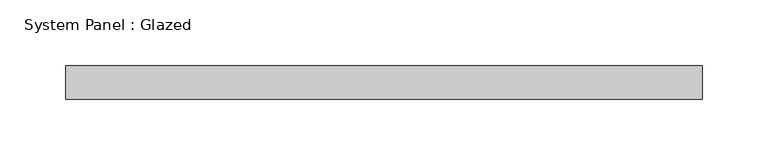
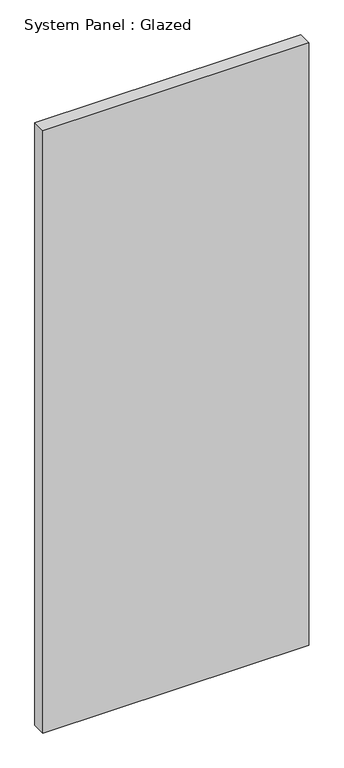
"""IFC4 building model written with IfcOpenShell, lengths in millimetres: plate geometry, System Panel : Glazed."""

from ifc_helpers import new_model, si_unit, origin, origin_with_axes, place, context, project, spatial, polyline, outline, extrude, source, transform, mapped, element, save


def system_panel_glazed_cd2dd794(model_context):
    return source(origin(), model_context, "Body", "SweptSolid", [
        extrude(outline(polyline([(241.3, 19.05), (-241.3, 19.05), (-241.3, 44.45), (241.3, 44.45), (241.3, 19.05)])), origin_with_axes(), (0.0, 0.0, 1.0), 1155.7),
    ])


if __name__ == "__main__":
    model = new_model("IFC4")
    model_context = context("Model", 3, world=origin())
    ifc_project = project(units=[si_unit("LENGTHUNIT", "METRE", prefix="MILLI")], contexts=[model_context])
    site = spatial("IfcSite", under=ifc_project)
    building = spatial("IfcBuilding", under=site)
    placement = place(None, origin())
    system_panel_glazed_shape = system_panel_glazed_cd2dd794(model_context)
    element("IfcPlate", 1, ObjectType="System Panel : Glazed", at=placement, inside=building, context=model_context, shape_type="MappedRepresentation", body=[
        mapped(system_panel_glazed_shape, transform((0.0, 0.0, 0.0), x_axis=(1.0, 0.0, 0.0), y_axis=(0.0, 1.0, 0.0), z_axis=(0.0, 0.0, 1.0))),
    ])
    save(model, "model.ifc")

# Revit data of these elements
# Type "System Panel : Glazed"
#   Construction Type Id = "GSP4R"
#   Analytic Construction = "1/8 in Pilkington single glazing"
#   Visual Light Transmittance = 0.9
#   Solar Heat Gain Coefficient = 0.86
#   Heat Transfer Coefficient (U) = 1.18115 BTU/(h·ft²·°F)
# Element 1 (IfcPlate, "System Panel : Glazed")
#   Materials on its faces: "Glass"
# Materials
#   "Glass": class "Glass", colour RGB 0 128 192, transparency 0.75, Description = "Soda Lime Glass", Cost = 0
